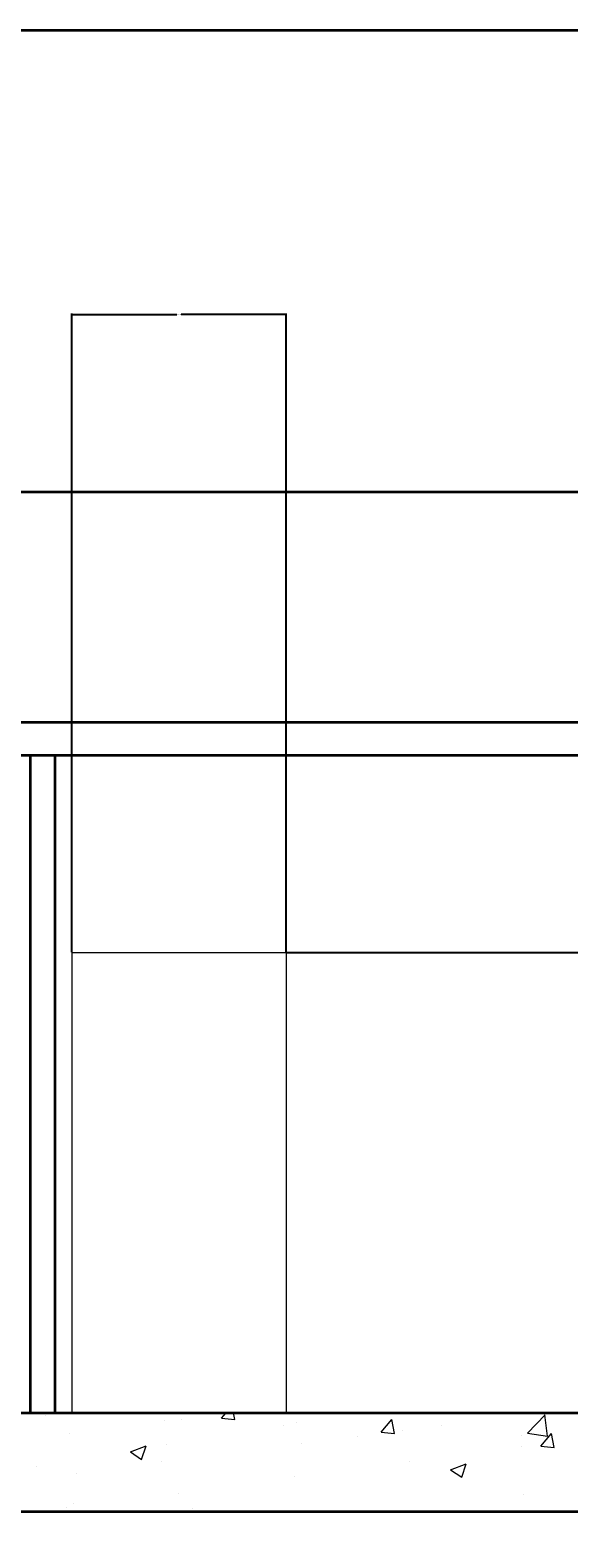
# Model space of a CAD drawing. Units: inches. Extents: x 2250 to 3547, y 1387 to 2604.
# Tile 8 of 11: x 3002 to 3100, y 2329 to 2604. Entities that reach past the tile are written whole.
import ezdxf

# ---------------------------------------------------------------- set-up
doc = ezdxf.new("R2010")
doc.units = ezdxf.units.IN
for name, color, linetype, lineweight in [('A-ANNO-DIMS', 2, 'Continuous', 18), ('A-ANNO-TTLB', 7, 'Continuous', 35), ('A-DOOR', 3, 'Continuous', 18), ('A-FLOR-PATT', 252, 'Continuous', 13), ('A-SECT', 7, 'Continuous', 35)]:
    doc.layers.add(name, color=color, linetype=linetype, lineweight=lineweight)
doc.styles.get("Standard").update_dxf_attribs({"font": 'arial.ttf'})
doc.dimstyles.get("Standard").update_dxf_attribs({"dimtxt": 0.18, "dimasz": 0.18, "dimexe": 0.18, "dimexo": 0.0625, "dimgap": 0.09, "dimtad": 0, "dimtih": 1, "dimtoh": 1, "dimdec": 4, "dimzin": 0, "dimdsep": 46, "dimtxsty": 'Standard', "dimcen": 0.09, "dimadec": 0, "dimazin": 0, "dimtfac": 1, "dimtdec": 4, "dimtofl": 0, "dimtmove": 0, "dimatfit": 3, "dimfxl": 1, "dimtolj": 1, "dimtzin": 0, "dimarcsym": 0})

# ---------------------------------------------------------------- blocks, each defined once
blk = doc.blocks.new('*D108')
at = {"layer": 'A-ANNO-DIMS', "color": 0, "lineweight": -2, "transparency": 16777216}
for p, q in [((2851.63, 2333.89), (2851.63, 2251.45)), ((3283.63, 2333.89), (3283.63, 2251.45)), ((2851.81, 2251.63), (3067.34, 2251.63)), ((3283.45, 2251.63), (3067.92, 2251.63))]:
    blk.add_line(p, q, dxfattribs=at)
at = {"layer": 'A-ANNO-DIMS', "color": 0, "transparency": 16777216}
for points in [[(2851.81, 2251.66), (2851.81, 2251.6), (2851.63, 2251.63)], [(3283.45, 2251.66), (3283.45, 2251.6), (3283.63, 2251.63)]]:
    blk.add_solid(points, dxfattribs=at)
at = {"layer": 'Defpoints', "color": 0, "transparency": 16777216}
for p in [(2851.63, 2333.95), (3283.63, 2333.95), (3283.63, 2251.63)]:
    blk.add_point(p, dxfattribs=at)
at = {"layer": 'A-ANNO-DIMS', "color": 0, "transparency": 16777216, "insert": (3067.63, 2251.63), "char_height": 0.18, "attachment_point": 5}
blk.add_mtext('\\A1;432', dxfattribs=at)
blk = doc.blocks.new('*D112')
at = {"layer": 'A-ANNO-DIMS', "color": 0, "lineweight": -2, "transparency": 16777216}
for p, q in [((3009.21, 2436.01), (3009.21, 2552.48)), ((3009.39, 2552.3), (3028.39, 2552.3)), ((3048.18, 2552.3), (3029.18, 2552.3)), ((3048.36, 2436.01), (3048.36, 2552.48))]:
    blk.add_line(p, q, dxfattribs=at)
at = {"layer": 'A-ANNO-DIMS', "color": 0, "transparency": 16777216}
for points in [[(3009.39, 2552.33), (3009.39, 2552.27), (3009.21, 2552.3)], [(3048.18, 2552.33), (3048.18, 2552.27), (3048.36, 2552.3)]]:
    blk.add_solid(points, dxfattribs=at)
at = {"layer": 'Defpoints', "color": 0, "transparency": 16777216}
for p in [(3048.36, 2552.3), (3009.21, 2435.95), (3048.36, 2435.95)]:
    blk.add_point(p, dxfattribs=at)
at = {"layer": 'A-ANNO-DIMS', "color": 0, "transparency": 16777216, "insert": (3028.79, 2552.3), "char_height": 0.18, "attachment_point": 5}
blk.add_mtext('\\A1;39.15', dxfattribs=at)
blk = doc.blocks.new('*D113')
at = {"layer": 'A-ANNO-DIMS', "color": 0, "lineweight": -2, "transparency": 16777216}
for p, q in [((3048.42, 2435.95), (3371.04, 2435.95)), ((3370.86, 2435.77), (3370.86, 2394.13)), ((3370.86, 2352.13), (3370.86, 2393.77)), ((3048.42, 2351.95), (3371.04, 2351.95))]:
    blk.add_line(p, q, dxfattribs=at)
at = {"layer": 'A-ANNO-DIMS', "color": 0, "transparency": 16777216}
for points in [[(3370.83, 2435.77), (3370.89, 2435.77), (3370.86, 2435.95)], [(3370.83, 2352.13), (3370.89, 2352.13), (3370.86, 2351.95)]]:
    blk.add_solid(points, dxfattribs=at)
at = {"layer": 'Defpoints', "color": 0, "transparency": 16777216}
for p in [(3048.36, 2435.95), (3370.86, 2435.95), (3048.36, 2351.95)]:
    blk.add_point(p, dxfattribs=at)
at = {"layer": 'A-ANNO-DIMS', "color": 0, "transparency": 16777216, "insert": (3370.86, 2393.95), "char_height": 0.18, "attachment_point": 5}
blk.add_mtext('\\A1;84', dxfattribs=at)

msp = doc.modelspace()

# ---------------------------------------------------------------- hatches: boundary and pattern name
at = {"layer": 'A-FLOR-PATT'}
h = msp.add_hatch(dxfattribs=at)
h.set_pattern_fill('AR-CONC', color=256, scale=0.16, style=0)
h.paths.add_polyline_path([(2851.6288, 2333.9493), (3283.6288, 2333.9493), (3283.6288, 2351.9493), (2851.6288, 2351.9493)])

# ---------------------------------------------------------------- linework, layer by layer
at = {"layer": 'A-ANNO-TTLB'}
msp.add_lwpolyline([(2250.1093, 2604.1988), (3546.995, 2604.1988), (3546.995, 1386.7251), (2250.1093, 1386.7251)], close=True, dxfattribs=at)
at = {"layer": 'A-DOOR'}
for p, q in [((3009.2144, 2435.9493), (3009.2144, 2351.9493)), ((3009.2144, 2435.9493), (3048.3624, 2435.9493)), ((3048.3624, 2435.9493), (3048.3624, 2351.9493))]:
    msp.add_line(p, q, dxfattribs=at)
at = {"layer": 'A-SECT'}
for p, q in [((2851.6288, 2519.9493), (3283.6288, 2519.9493)), ((2851.6288, 2477.9493), (3283.6288, 2477.9493)), ((2851.6288, 2471.9493), (3283.6288, 2471.9493)), ((3001.6288, 2471.9493), (3001.6288, 2351.9493)), ((3006.1288, 2471.9493), (3006.1288, 2351.9493)), ((2851.6288, 2351.9493), (3283.6288, 2351.9493)), ((2851.6288, 2333.9493), (3283.6288, 2333.9493))]:
    msp.add_line(p, q, dxfattribs=at)

# ---------------------------------------------------------------- dimensions: what is measured, and where the dimension line sits
at = {"layer": 'A-ANNO-DIMS'}
for base, p1, p2, override, picture, middle in [((3048.3624, 2552.2993), (3009.2144, 2435.9493), (3048.3624, 2435.9493), {"dimdec": 2, "dimlfac": 1, "dimrnd": 0, "dimzin": 0, "dimdsep": 46, "dimlunit": 2}, '*D112', (3028.7884, 2552.2993)), ((3283.6288, 2251.631), (2851.6288, 2333.9493), (3283.6288, 2333.9493), {"dimdec": 0, "dimlfac": 1, "dimrnd": 0, "dimzin": 0, "dimdsep": 46, "dimlunit": 2}, '*D108', (3067.6288, 2251.631))]:
    dim = msp.add_linear_dim(base=base, p1=p1, p2=p2, dimstyle='Standard', override=override, dxfattribs=at)
    dim.commit()
    dim.dimension.update_dxf_attribs({"geometry": picture, "text_midpoint": middle})
dim = msp.add_linear_dim(base=(3370.8583, 2435.9493), p1=(3048.3624, 2351.9493), p2=(3048.3624, 2435.9493), angle=90, dimstyle='Standard', override={"dimdec": 0, "dimlfac": 1, "dimrnd": 0, "dimzin": 0, "dimdsep": 46, "dimlunit": 2}, dxfattribs=at)
dim.commit()
dim.dimension.update_dxf_attribs({"geometry": '*D113', "text_midpoint": (3370.8583, 2393.9493)})

doc.saveas('drawing.dxf')
